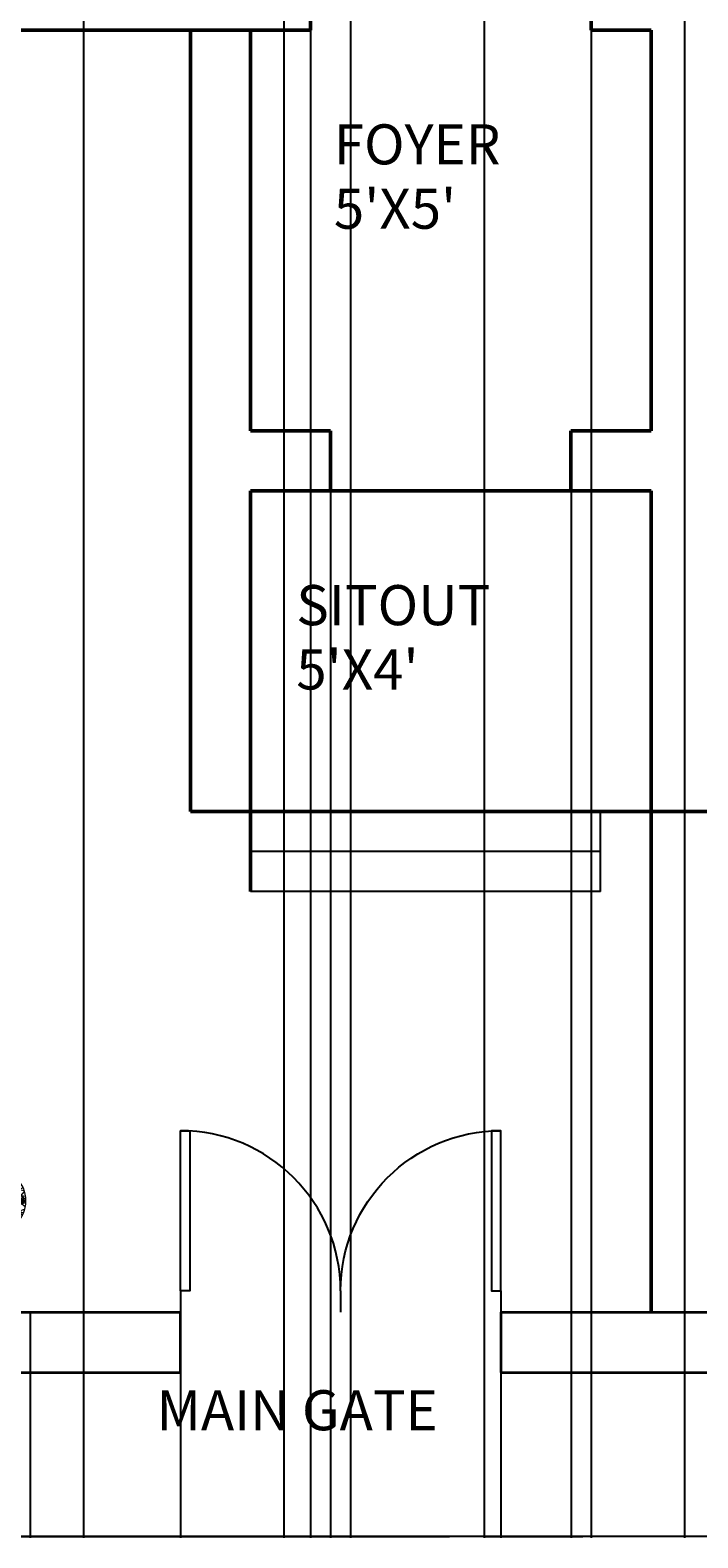
# Model space of a CAD drawing. Units: inches. Extents: x 8049 to 8459, y 820 to 1350.
# Tile 19 of 25: x 8197 to 8297, y 820 to 1046. Entities that reach past the tile are written whole.
import ezdxf

# ---------------------------------------------------------------- set-up
doc = ezdxf.new("R2010")
doc.units = ezdxf.units.IN
doc.header["$MEASUREMENT"] = 0
for name, color, linetype, lineweight in [('A-ANNO-DIMS', 2, 'Continuous', 18), ('A-ANNO-TEXT', 7, 'Continuous', 18), ('A-AREA-IDEN', 7, 'Continuous', 25), ('A-FLOR-STRS', 7, 'Continuous', 25), ('A-WALL', 7, 'Continuous', 50), ('C-SITE-GATE', 3, 'Continuous', 25), ('C-SITE-WALL', 7, 'Continuous', 35), ('zelen', 69, 'Continuous', 13)]:
    doc.layers.add(name, color=color, linetype=linetype, lineweight=lineweight)
doc.styles.get("Standard").update_dxf_attribs({"font": 'arial.ttf'})
doc.dimstyles.get("Standard").update_dxf_attribs({"dimtxt": 0.18, "dimasz": 0.18, "dimexe": 0.18, "dimexo": 0.0625, "dimgap": 0.09, "dimtad": 0, "dimtih": 1, "dimtoh": 1, "dimdec": 4, "dimzin": 0, "dimdsep": 46, "dimtxsty": 'Standard', "dimcen": 0.09, "dimadec": 0, "dimazin": 0, "dimtfac": 1, "dimtdec": 4, "dimtofl": 0, "dimtmove": 0, "dimatfit": 3, "dimfxl": 1, "dimtolj": 1, "dimtzin": 0, "dimarcsym": 0})

# ---------------------------------------------------------------- blocks, each defined once
blk = doc.blocks.new('*U2')
for p, q in [((0, 0), (0, -100)), ((750, 0), (750, -100))]:
    blk.add_line(p, q)
blk.add_lwpolyline([(0, 0), (0, 750), (43.75, 750), (43.75, 0)], close=True)
blk.add_arc((0, 0), 750, 0, 90)
blk = doc.blocks.new('T40C')
for p, q in [((-0.237, 0.384), (-0.221, 0.459)), ((-0.133, 0.438), (-0.217, 0.461)), ((-0.005, 0.298), (-0.171, 0.48)), ((-0.122, 0.426), (-0.113, 0.5)), ((-0.002, 0.444), (-0.055, 0.507)), ((-0.002, 0.014), (-0.002, 0.511)), ((-0.002, 0.511), (-0.002, -0.477)), ((-0.002, 0.436), (0.059, 0.505)), ((-0.002, 0.289), (0.139, 0.49)), ((0.104, 0.44), (0.075, 0.504)), ((0.098, 0.431), (0.181, 0.475)), ((0.222, 0.407), (0.185, 0.476)), ((0.209, 0.224), (0.225, 0.457)), ((-0.377, 0.251), (-0.449, 0.228)), ((-0.203, 0.214), (-0.433, 0.263)), ((-0.384, 0.252), (-0.408, 0.298)), ((-0.305, 0.323), (-0.389, 0.323)), ((0.351, 0.366), (-0.349, -0.333)), ((0.001, 0.016), (-0.344, 0.362)), ((-0.344, 0.362), (0.346, -0.329)), ((-0.304, 0.322), (-0.313, 0.4)), ((-0.237, 0.382), (-0.298, 0.412)), ((-0.2, 0.218), (-0.251, 0.446)), ((-0.002, 0.014), (0.105, 0.438)), ((-0.002, 0.014), (0.117, 0.433)), ((-0.002, 0.014), (0.203, 0.413)), ((-0.002, 0.014), (0.085, 0.408)), ((-0.002, 0.014), (0.207, 0.357)), ((-0.002, 0.014), (0.199, 0.293)), ((-0.002, 0.014), (0.184, 0.238)), ((0.001, 0.016), (0.142, 0.435)), ((0.001, 0.016), (0.18, 0.434)), ((0.001, 0.016), (0.161, 0.432)), ((0.001, 0.016), (0.351, 0.366)), ((0.001, 0.016), (0.049, 0.337)), ((0.001, 0.016), (0.017, 0.302)), ((0.209, 0.225), (0.442, 0.236)), ((0.221, 0.393), (0.288, 0.417)), ((0.298, 0.313), (0.313, 0.399)), ((0.301, 0.316), (0.38, 0.331)), ((0.385, 0.234), (0.405, 0.298)), ((0.386, 0.234), (0.46, 0.196)), ((0.391, 0.234), (0.398, 0.234)), ((-0.442, 0.014), (-0.497, 0.063)), ((-0.428, 0.014), (-0.495, -0.044)), ((0.495, 0.014), (-0.494, 0.014)), ((-0.428, 0.125), (-0.49, 0.101)), ((-0.295, 0.014), (-0.474, 0.163)), ((-0.285, 0.017), (-0.472, -0.143)), ((-0.428, 0.125), (-0.46, 0.209)), ((-0.002, 0.014), (-0.448, -0.156)), ((-0.002, 0.014), (-0.446, -0.131)), ((-0.002, 0.014), (-0.442, -0.143)), ((-0.002, 0.014), (-0.438, -0.174)), ((-0.002, 0.014), (-0.433, -0.112)), ((-0.002, 0.014), (-0.432, -0.186)), ((-0.432, -0.186), (-0.002, 0.014)), ((-0.002, 0.014), (-0.415, -0.097)), ((-0.002, 0.014), (-0.401, -0.195)), ((-0.002, 0.014), (-0.386, -0.077)), ((-0.002, 0.014), (-0.365, -0.059)), ((-0.002, 0.014), (-0.359, -0.197)), ((-0.002, 0.014), (-0.331, -0.03)), ((-0.002, 0.014), (-0.316, -0.015)), ((-0.002, 0.014), (-0.301, -0.004)), ((-0.002, 0.014), (-0.292, 0.006)), ((-0.002, 0.014), (-0.286, -0.186)), ((-0.002, 0.014), (-0.231, -0.181)), ((-0.002, 0.014), (-0.053, -0.002)), ((-0.002, 0.014), (-0.053, -0.002)), ((-0.002, 0.014), (0.001, 0.016)), ((-0.002, 0.014), (0.495, 0.014)), ((-0.002, 0.014), (0.009, -0.267)), ((-0.002, 0.014), (0.024, -0.277)), ((-0.002, 0.014), (0.041, -0.303)), ((-0.002, 0.014), (0.063, -0.324)), ((-0.002, 0.014), (0.087, -0.352)), ((-0.002, 0.014), (0.11, -0.388)), ((-0.002, 0.014), (0.134, -0.406)), ((-0.002, 0.014), (0.152, -0.42)), ((-0.002, 0.014), (0.167, -0.421)), ((-0.002, 0.014), (0.18, -0.42)), ((-0.002, 0.014), (0.196, -0.42)), ((-0.002, 0.014), (0.201, -0.395)), ((-0.002, 0.014), (0.207, -0.383)), ((-0.002, 0.014), (0.206, -0.365)), ((-0.002, 0.014), (0.202, -0.323)), ((-0.002, 0.014), (0.204, -0.305)), ((-0.002, 0.014), (0.204, -0.281)), ((-0.002, 0.014), (0.198, -0.25)), ((-0.002, 0.014), (0.197, -0.233)), ((-0.002, 0.014), (0.201, -0.217)), ((-0.002, 0.014), (0.196, -0.196)), ((0.285, 0.014), (0.472, -0.133)), ((0.292, 0.014), (0.375, 0.014)), ((0.294, 0.014), (0.474, 0.156)), ((0.426, 0.118), (0.459, 0.199)), ((0.429, 0.12), (0.487, 0.098)), ((0.431, 0.014), (0.491, 0.068)), ((0.435, 0.017), (0.493, -0.028)), ((-0.429, -0.107), (-0.487, -0.086)), ((-0.439, -0.115), (-0.459, -0.178)), ((-0.053, -0.002), (-0.455, -0.166)), ((-0.371, -0.219), (-0.453, -0.192)), ((-0.207, -0.191), (-0.434, -0.23)), ((-0.371, -0.219), (-0.395, -0.287)), ((-0.053, -0.002), (-0.346, -0.045)), ((-0.207, -0.191), (-0.241, -0.42)), ((0.204, -0.187), (0.215, -0.433)), ((0.207, -0.19), (0.432, -0.224)), ((0.363, -0.213), (0.448, -0.197)), ((0.375, -0.215), (0.393, -0.287)), ((0.419, -0.091), (0.483, -0.091)), ((0.422, -0.093), (0.453, -0.184)), ((-0.313, -0.294), (-0.384, -0.302)), ((-0.312, -0.297), (-0.308, -0.376)), ((-0.232, -0.36), (-0.29, -0.388)), ((-0.231, -0.355), (-0.203, -0.439)), ((-0.105, -0.406), (-0.192, -0.443)), ((-0.002, -0.26), (-0.142, -0.46)), ((-0.109, -0.412), (-0.087, -0.473)), ((-0.002, -0.414), (-0.047, -0.478)), ((-0.002, -0.256), (0.16, -0.453)), ((-0.002, -0.411), (0.051, -0.477)), ((0.117, -0.401), (0.095, -0.473)), ((0.126, -0.411), (0.186, -0.443)), ((0.212, -0.374), (0.188, -0.442)), ((0.212, -0.367), (0.272, -0.397)), ((0.301, -0.283), (0.387, -0.291)), ((0.301, -0.285), (0.302, -0.379))]:
    blk.add_line(p, q)
blk.add_circle((-0.002, 0.014), 0.496)
blk = doc.blocks.new('*D53')
at = {"layer": 'A-ANNO-DIMS', "color": 0, "lineweight": -2, "transparency": 16777216}
for p, q in [((8197.4, 853.81), (8197.4, 820.09)), ((8219.9, 853.81), (8219.9, 820.09)), ((8197.58, 820.27), (8208.32, 820.27)), ((8219.72, 820.27), (8208.97, 820.27))]:
    blk.add_line(p, q, dxfattribs=at)
at = {"layer": 'A-ANNO-DIMS', "color": 0, "transparency": 16777216}
for points in [[(8197.58, 820.3), (8197.58, 820.24), (8197.4, 820.27)], [(8219.72, 820.3), (8219.72, 820.24), (8219.9, 820.27)]]:
    blk.add_solid(points, dxfattribs=at)
at = {"layer": 'Defpoints', "color": 0, "transparency": 16777216}
for p in [(8197.4, 853.87), (8219.9, 853.87), (8219.9, 820.27)]:
    blk.add_point(p, dxfattribs=at)
at = {"layer": 'A-ANNO-DIMS', "color": 0, "transparency": 16777216, "insert": (8208.65, 820.27), "char_height": 0.18, "attachment_point": 5}
blk.add_mtext('\\A1;22.5', dxfattribs=at)
blk = doc.blocks.new('*D54')
at = {"layer": 'A-ANNO-DIMS', "color": 0, "lineweight": -2, "transparency": 16777216}
for p, q in [((8219.9, 844.81), (8219.9, 820.09)), ((8267.9, 844.81), (8267.9, 820.09)), ((8220.08, 820.27), (8243.67, 820.27)), ((8267.72, 820.27), (8244.12, 820.27))]:
    blk.add_line(p, q, dxfattribs=at)
at = {"layer": 'A-ANNO-DIMS', "color": 0, "transparency": 16777216}
for points in [[(8220.08, 820.3), (8220.08, 820.24), (8219.9, 820.27)], [(8267.72, 820.3), (8267.72, 820.24), (8267.9, 820.27)]]:
    blk.add_solid(points, dxfattribs=at)
at = {"layer": 'Defpoints', "color": 0, "transparency": 16777216}
for p in [(8219.9, 844.87), (8267.9, 844.87), (8267.9, 820.27)]:
    blk.add_point(p, dxfattribs=at)
at = {"layer": 'A-ANNO-DIMS', "color": 0, "transparency": 16777216, "insert": (8243.9, 820.27), "char_height": 0.18, "attachment_point": 5}
blk.add_mtext('\\A1;48', dxfattribs=at)
blk = doc.blocks.new('*D55')
at = {"layer": 'A-ANNO-DIMS', "color": 0, "lineweight": -2, "transparency": 16777216}
for p, q in [((8239.4, 1045.81), (8239.4, 820.09)), ((8281.4, 1045.81), (8281.4, 820.09)), ((8239.58, 820.27), (8260.18, 820.27)), ((8281.22, 820.27), (8260.62, 820.27))]:
    blk.add_line(p, q, dxfattribs=at)
at = {"layer": 'A-ANNO-DIMS', "color": 0, "transparency": 16777216}
for points in [[(8239.58, 820.3), (8239.58, 820.24), (8239.4, 820.27)], [(8281.22, 820.3), (8281.22, 820.24), (8281.4, 820.27)]]:
    blk.add_solid(points, dxfattribs=at)
at = {"layer": 'Defpoints', "color": 0, "transparency": 16777216}
for p in [(8239.4, 1045.87), (8281.4, 1045.87), (8281.4, 820.27)]:
    blk.add_point(p, dxfattribs=at)
at = {"layer": 'A-ANNO-DIMS', "color": 0, "transparency": 16777216, "insert": (8260.4, 820.27), "char_height": 0.18, "attachment_point": 5}
blk.add_mtext('\\A1;42', dxfattribs=at)
blk = doc.blocks.new('*D56')
at = {"layer": 'A-ANNO-DIMS', "color": 0, "lineweight": -2, "transparency": 16777216}
for p, q in [((8205.4, 1156.81), (8205.4, 820.09)), ((8235.4, 1156.81), (8235.4, 820.09)), ((8205.58, 820.27), (8220.18, 820.27)), ((8235.22, 820.27), (8220.62, 820.27))]:
    blk.add_line(p, q, dxfattribs=at)
at = {"layer": 'A-ANNO-DIMS', "color": 0, "transparency": 16777216}
for points in [[(8205.58, 820.3), (8205.58, 820.24), (8205.4, 820.27)], [(8235.22, 820.3), (8235.22, 820.24), (8235.4, 820.27)]]:
    blk.add_solid(points, dxfattribs=at)
at = {"layer": 'Defpoints', "color": 0, "transparency": 16777216}
for p in [(8205.4, 1156.87), (8235.4, 1156.87), (8235.4, 820.27)]:
    blk.add_point(p, dxfattribs=at)
at = {"layer": 'A-ANNO-DIMS', "color": 0, "transparency": 16777216, "insert": (8220.4, 820.27), "char_height": 0.18, "attachment_point": 5}
blk.add_mtext('\\A1;30', dxfattribs=at)
blk = doc.blocks.new('*D61')
at = {"layer": 'A-ANNO-DIMS', "color": 0, "lineweight": -2, "transparency": 16777216}
for p, q in [((8242.4, 976.81), (8242.4, 820.09)), ((8278.4, 976.81), (8278.4, 820.09)), ((8242.58, 820.27), (8260.18, 820.27)), ((8278.22, 820.27), (8260.62, 820.27))]:
    blk.add_line(p, q, dxfattribs=at)
at = {"layer": 'A-ANNO-DIMS', "color": 0, "transparency": 16777216}
for points in [[(8242.58, 820.3), (8242.58, 820.24), (8242.4, 820.27)], [(8278.22, 820.3), (8278.22, 820.24), (8278.4, 820.27)]]:
    blk.add_solid(points, dxfattribs=at)
at = {"layer": 'Defpoints', "color": 0, "transparency": 16777216}
for p in [(8242.4, 976.87), (8278.4, 976.87), (8278.4, 820.27)]:
    blk.add_point(p, dxfattribs=at)
at = {"layer": 'A-ANNO-DIMS', "color": 0, "transparency": 16777216, "insert": (8260.4, 820.27), "char_height": 0.18, "attachment_point": 5}
blk.add_mtext('\\A1;36', dxfattribs=at)
blk = doc.blocks.new('*D71')
at = {"layer": 'A-ANNO-DIMS', "color": 0, "lineweight": -2, "transparency": 16777216}
for p, q in [((8185.4, 1045.81), (8185.4, 820.09)), ((8239.4, 1045.81), (8239.4, 820.09)), ((8185.58, 820.27), (8212.18, 820.27)), ((8239.22, 820.27), (8212.62, 820.27))]:
    blk.add_line(p, q, dxfattribs=at)
at = {"layer": 'A-ANNO-DIMS', "color": 0, "transparency": 16777216}
for points in [[(8185.58, 820.3), (8185.58, 820.24), (8185.4, 820.27)], [(8239.22, 820.3), (8239.22, 820.24), (8239.4, 820.27)]]:
    blk.add_solid(points, dxfattribs=at)
at = {"layer": 'Defpoints', "color": 0, "transparency": 16777216}
for p in [(8185.4, 1045.87), (8239.4, 1045.87), (8239.4, 820.27)]:
    blk.add_point(p, dxfattribs=at)
at = {"layer": 'A-ANNO-DIMS', "color": 0, "transparency": 16777216, "insert": (8212.4, 820.27), "char_height": 0.18, "attachment_point": 5}
blk.add_mtext('\\A1;54', dxfattribs=at)
blk = doc.blocks.new('*D73')
at = {"layer": 'A-ANNO-DIMS', "color": 0, "lineweight": -2, "transparency": 16777216}
for p, q in [((8239.4, 1204.81), (8239.4, 820.09)), ((8265.4, 1204.81), (8265.4, 820.09)), ((8239.58, 820.27), (8252.18, 820.27)), ((8265.22, 820.27), (8252.62, 820.27))]:
    blk.add_line(p, q, dxfattribs=at)
at = {"layer": 'A-ANNO-DIMS', "color": 0, "transparency": 16777216}
for points in [[(8239.58, 820.3), (8239.58, 820.24), (8239.4, 820.27)], [(8265.22, 820.3), (8265.22, 820.24), (8265.4, 820.27)]]:
    blk.add_solid(points, dxfattribs=at)
at = {"layer": 'Defpoints', "color": 0, "transparency": 16777216}
for p in [(8239.4, 1204.87), (8265.4, 1204.87), (8265.4, 820.27)]:
    blk.add_point(p, dxfattribs=at)
at = {"layer": 'A-ANNO-DIMS', "color": 0, "transparency": 16777216, "insert": (8252.4, 820.27), "char_height": 0.18, "attachment_point": 5}
blk.add_mtext('\\A1;26', dxfattribs=at)
blk = doc.blocks.new('*D75')
at = {"layer": 'A-ANNO-DIMS', "color": 0, "lineweight": -2, "transparency": 16777216}
for p, q in [((8239.4, 1162.81), (8239.4, 820.09)), ((8245.4, 1156.81), (8245.4, 820.09)), ((8239.58, 820.27), (8242.25, 820.27)), ((8245.22, 820.27), (8242.55, 820.27))]:
    blk.add_line(p, q, dxfattribs=at)
at = {"layer": 'A-ANNO-DIMS', "color": 0, "transparency": 16777216}
for points in [[(8239.58, 820.3), (8239.58, 820.24), (8239.4, 820.27)], [(8245.22, 820.3), (8245.22, 820.24), (8245.4, 820.27)]]:
    blk.add_solid(points, dxfattribs=at)
at = {"layer": 'Defpoints', "color": 0, "transparency": 16777216}
for p in [(8239.4, 1162.87), (8245.4, 1156.87), (8245.4, 820.27)]:
    blk.add_point(p, dxfattribs=at)
at = {"layer": 'A-ANNO-DIMS', "color": 0, "transparency": 16777216, "insert": (8242.4, 820.27), "char_height": 0.18, "attachment_point": 5}
blk.add_mtext('\\A1;6', dxfattribs=at)
blk = doc.blocks.new('*D76')
at = {"layer": 'A-ANNO-DIMS', "color": 0, "lineweight": -2, "transparency": 16777216}
for p, q in [((8083.4, 1054.81), (8083.4, 820.09)), ((8299.4, 1054.81), (8299.4, 820.09)), ((8083.58, 820.27), (8191.11, 820.27)), ((8299.22, 820.27), (8191.69, 820.27))]:
    blk.add_line(p, q, dxfattribs=at)
at = {"layer": 'A-ANNO-DIMS', "color": 0, "transparency": 16777216}
for points in [[(8083.58, 820.3), (8083.58, 820.24), (8083.4, 820.27)], [(8299.22, 820.3), (8299.22, 820.24), (8299.4, 820.27)]]:
    blk.add_solid(points, dxfattribs=at)
at = {"layer": 'Defpoints', "color": 0, "transparency": 16777216}
for p in [(8083.4, 1054.87), (8299.4, 1054.87), (8299.4, 820.27)]:
    blk.add_point(p, dxfattribs=at)
at = {"layer": 'A-ANNO-DIMS', "color": 0, "transparency": 16777216, "insert": (8191.4, 820.27), "char_height": 0.18, "attachment_point": 5}
blk.add_mtext('\\A1;216', dxfattribs=at)
blk = doc.blocks.new('*D86')
at = {"layer": 'A-ANNO-DIMS', "color": 0, "lineweight": -2, "transparency": 16777216}
for p, q in [((8265.4, 1204.81), (8265.4, 820.09)), ((8295.4, 1204.81), (8295.4, 820.09)), ((8265.58, 820.27), (8280.18, 820.27)), ((8295.22, 820.27), (8280.62, 820.27))]:
    blk.add_line(p, q, dxfattribs=at)
at = {"layer": 'A-ANNO-DIMS', "color": 0, "transparency": 16777216}
for points in [[(8265.58, 820.3), (8265.58, 820.24), (8265.4, 820.27)], [(8295.22, 820.3), (8295.22, 820.24), (8295.4, 820.27)]]:
    blk.add_solid(points, dxfattribs=at)
at = {"layer": 'Defpoints', "color": 0, "transparency": 16777216}
for p in [(8265.4, 1204.87), (8295.4, 1204.87), (8295.4, 820.27)]:
    blk.add_point(p, dxfattribs=at)
at = {"layer": 'A-ANNO-DIMS', "color": 0, "transparency": 16777216, "insert": (8280.4, 820.27), "char_height": 0.18, "attachment_point": 5}
blk.add_mtext('\\A1;30', dxfattribs=at)

msp = doc.modelspace()

# ---------------------------------------------------------------- linework, layer by layer
at = {"layer": 'A-FLOR-STRS'}
for p, q in [((8282.798, 916.8706), (8282.798, 928.8706)), ((8282.798, 922.8706), (8230.3974, 922.8706)), ((8282.798, 916.8706), (8230.3974, 916.8706))]:
    msp.add_line(p, q, dxfattribs=at)
at = {"layer": 'A-WALL'}
for p, q in [((8239.3974, 1045.8706), (8239.3974, 1054.8706)), ((8281.3974, 1054.8706), (8281.3974, 1045.8706)), ((8083.3974, 1045.8706), (8239.3974, 1045.8706)), ((8221.3974, 928.8706), (8221.3974, 1045.8706)), ((8230.3974, 985.8706), (8230.3974, 1045.8706)), ((8281.3974, 1045.8706), (8290.3974, 1045.8706)), ((8290.3974, 985.8706), (8290.3974, 1045.8706)), ((8242.3974, 985.8706), (8230.3974, 985.8706)), ((8242.3974, 976.8706), (8242.3974, 985.8706)), ((8290.3974, 985.8706), (8278.3974, 985.8706)), ((8278.3974, 985.8706), (8278.3974, 976.8706)), ((8230.3974, 916.8706), (8230.3974, 976.8706)), ((8290.3974, 976.8706), (8230.3974, 976.8706)), ((8290.3974, 853.8706), (8290.3974, 976.8706)), ((8299.3974, 928.8706), (8221.3974, 928.8706))]:
    msp.add_line(p, q, dxfattribs=at)
at = {"layer": 'C-SITE-WALL'}
for p, q in [((8083.3974, 853.8706), (8219.8974, 853.8706)), ((8219.8974, 844.8706), (8219.8974, 853.8706)), ((8267.8765, 853.8706), (8425.3974, 853.8706)), ((8267.8974, 853.8706), (8267.8974, 844.8706)), ((8074.3974, 844.8706), (8219.8974, 844.8706)), ((8267.8974, 844.8706), (8434.3974, 844.8706))]:
    msp.add_line(p, q, dxfattribs=at)

# ---------------------------------------------------------------- block references
at = {"layer": 'C-SITE-GATE', "yscale": 0.0319860725682742, "zscale": 0.0319860725682742}
for p, xscale in [((8219.8974, 857.0692), 0.0319860725682742), ((8267.8765, 857.0692), -0.0319860725682742)]:
    msp.add_blockref('*U2', p, dxfattribs=dict(at, xscale=xscale))
at = {"layer": 'zelen', "xscale": 9.920223989974332, "yscale": 9.920223989974332, "zscale": 9.920223989974332, "rotation": 158.4000000000004}
msp.add_blockref('T40C', (8191.8288, 870.7033), dxfattribs=at)

# ---------------------------------------------------------------- texts
at = {"layer": 'A-ANNO-TEXT'}
msp.add_text('MAIN GATE', height=6, dxfattribs=at).set_placement((8216.334, 836.2004))
at = {"layer": 'A-AREA-IDEN'}
for s, p in [('FOYER', (8242.8846, 1025.7678)), ("5'X5'", (8242.8846, 1016.1294)), ('SITOUT', (8237.2559, 956.7647)), ("5'X4'", (8237.2559, 947.1262))]:
    msp.add_text(s, height=6, dxfattribs=at).set_placement(p)

# ---------------------------------------------------------------- dimensions: what is measured, and where the dimension line sits
at = {"layer": 'A-ANNO-DIMS'}
for base, p1, p2, override, picture, middle in [((8265.3974, 820.2706), (8239.3974, 1204.8706), (8265.3974, 1204.8706), {"dimdec": 0, "dimlfac": 1, "dimrnd": 0, "dimzin": 0, "dimdsep": 46, "dimlunit": 2}, '*D73', (8252.3974, 820.2706)), ((8295.3974, 820.2706), (8265.3974, 1204.8706), (8295.3974, 1204.8706), {"dimdec": 0, "dimlfac": 1, "dimrnd": 0, "dimzin": 0, "dimdsep": 46, "dimlunit": 2}, '*D86', (8280.3974, 820.2706)), ((8245.3974, 820.2706), (8239.3974, 1162.8706), (8245.3974, 1156.8706), {"dimdec": 0, "dimlfac": 1, "dimrnd": 0, "dimzin": 0, "dimdsep": 46, "dimlunit": 2}, '*D75', (8242.3974, 820.2706)), ((8235.3974, 820.2706), (8205.3974, 1156.8706), (8235.3974, 1156.8706), {"dimdec": 0, "dimlfac": 1, "dimrnd": 0, "dimzin": 0, "dimdsep": 46, "dimlunit": 2}, '*D56', (8220.3974, 820.2706)), ((8299.3974, 820.2706), (8083.3974, 1054.8706), (8299.3974, 1054.8706), {"dimdec": 0, "dimlfac": 1, "dimrnd": 0, "dimzin": 0, "dimdsep": 46, "dimlunit": 2}, '*D76', (8191.3974, 820.2706)), ((8239.3974, 820.2706), (8185.3974, 1045.8706), (8239.3974, 1045.8706), {"dimdec": 0, "dimlfac": 1, "dimrnd": 0, "dimzin": 0, "dimdsep": 46, "dimlunit": 2}, '*D71', (8212.3974, 820.2706)), ((8281.3974, 820.2706), (8239.3974, 1045.8706), (8281.3974, 1045.8706), {"dimdec": 0, "dimlfac": 1, "dimrnd": 0, "dimzin": 0, "dimdsep": 46, "dimlunit": 2}, '*D55', (8260.3974, 820.2706)), ((8278.3974, 820.2706), (8242.3974, 976.8706), (8278.3974, 976.8706), {"dimdec": 0, "dimlfac": 1, "dimrnd": 0, "dimzin": 0, "dimdsep": 46, "dimlunit": 2}, '*D61', (8260.3974, 820.2706)), ((8219.8974, 820.2706), (8197.3974, 853.8706), (8219.8974, 853.8706), {"dimdec": 1, "dimlfac": 1, "dimrnd": 0, "dimzin": 0, "dimdsep": 46, "dimlunit": 2}, '*D53', (8208.6474, 820.2706)), ((8267.8974, 820.2706), (8219.8974, 844.8706), (8267.8974, 844.8706), {"dimdec": 0, "dimlfac": 1, "dimrnd": 0, "dimzin": 0, "dimdsep": 46, "dimlunit": 2}, '*D54', (8243.8974, 820.2706))]:
    dim = msp.add_linear_dim(base=base, p1=p1, p2=p2, dimstyle='Standard', override=override, dxfattribs=at)
    dim.commit()
    dim.dimension.update_dxf_attribs({"geometry": picture, "text_midpoint": middle})

doc.saveas('drawing.dxf')
